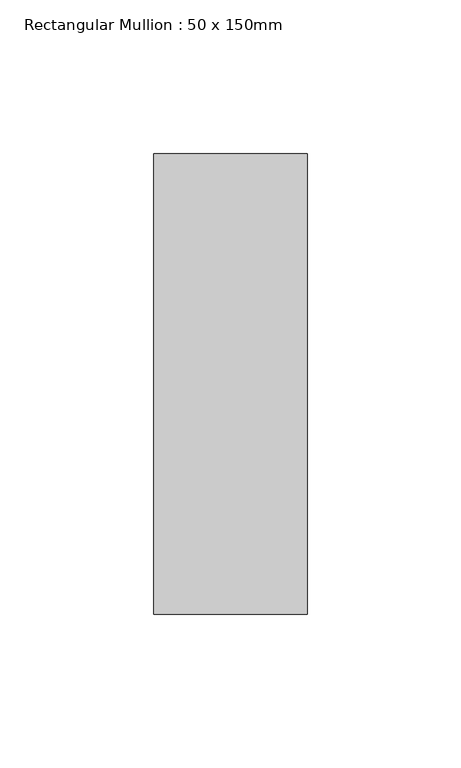
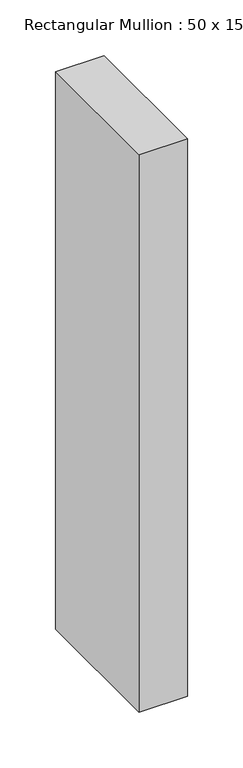
"""IFC4 building model written with IfcOpenShell, lengths in millimetres: member geometry, Rectangular Mullion : 50 x 150mm."""

from ifc_helpers import new_model, si_unit, frame, origin, place, context, project, spatial, polyline, outline, extrude, source, transform, mapped, element, save


def rectangular_mullion_50_x_150mm_de2b7ee4(model_context):
    return source(origin(), model_context, "Body", "SweptSolid", [
        extrude(outline(polyline([(25.0, 75.0), (25.0, -75.0), (-25.0, -75.0), (-25.0, 75.0), (25.0, 75.0)])), frame((0.0, 0.0, -610.0), z_axis=(0.0, 0.0, 1.0), x_axis=(1.0, 0.0, 0.0)), (0.0, 0.0, 1.0), 610.0),
    ])


if __name__ == "__main__":
    model = new_model("IFC4")
    model_context = context("Model", 3, world=origin())
    ifc_project = project(units=[si_unit("LENGTHUNIT", "METRE", prefix="MILLI")], contexts=[model_context])
    site = spatial("IfcSite", under=ifc_project)
    building = spatial("IfcBuilding", under=site)
    placement = place(None, origin())
    rectangular_mullion_50_x_150mm_shape = rectangular_mullion_50_x_150mm_de2b7ee4(model_context)
    element("IfcMember", 1, ObjectType="Rectangular Mullion : 50 x 150mm", at=placement, inside=building, context=model_context, shape_type="MappedRepresentation", body=[
        mapped(rectangular_mullion_50_x_150mm_shape, transform((0.0, 0.0, 0.0), x_axis=(1.0, 0.0, 0.0), y_axis=(0.0, 1.0, 0.0), z_axis=(0.0, 0.0, 1.0))),
    ])
    save(model, "model.ifc")

# Revit data of these elements
# Type "Rectangular Mullion : 50 x 150mm"
#   built-in parameter 1007304 = 0.492126 (stored number, unit not read)
#   built-in parameter 1007301 = 0.082021 (stored number, unit not read)
#   built-in parameter 1007300 = 0.082021 (stored number, unit not read)
# Element 1 (IfcMember, "Rectangular Mullion : 50 x 150mm")
#   Materials on its faces: "Aluminium"
# Materials
#   "Aluminium": class "Metal", colour RGB 247 247 247, transparency 0, Description = "Aluminium 6061", Cost = 0
